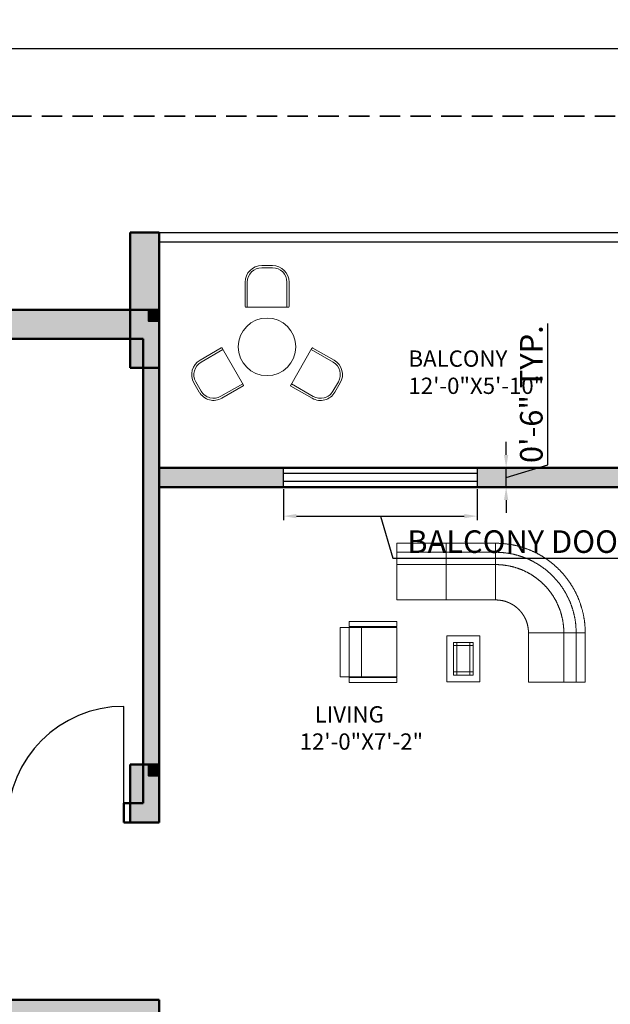
# Model space of a CAD drawing. Units: inches. Extents: x -7 to 1228, y -146 to 1091.
# Tile 57 of 88: x 193 to 376, y 786 to 1091. Entities that reach past the tile are written whole.
import ezdxf

# ---------------------------------------------------------------- set-up
doc = ezdxf.new("R2010")
doc.units = ezdxf.units.IN
doc.linetypes.add('DASHED2', pattern=[9.525, 6.35, -3.175])
for name, color, linetype, lineweight in [('A-ANNO-DIMS', 2, 'Continuous', 18), ('A-AREA-IDEN', 7, 'Continuous', 18), ('A-COLS', 6, 'Continuous', 35), ('A-DOOR', 4, 'Continuous', 25), ('A-FURN', 8, 'Continuous', 18), ('A-GLAZ', 175, 'Continuous', 25), ('A-WALL', 7, 'Continuous', 50), ('A-WALL-PATT', 251, 'Continuous', 13), ('C-PROP', 1, 'DASHED2', 35)]:
    doc.layers.add(name, color=color, linetype=linetype, lineweight=lineweight)
doc.styles.get("Standard").update_dxf_attribs({"font": 'arial.ttf'})
doc.dimstyles.new('ISO-25', dxfattribs={"dimtxt": 7, "dimasz": 4, "dimexe": 1.25, "dimexo": 0.625, "dimtad": 1, "dimdec": 1, "dimlunit": 3, "dimtxsty": 'Standard', "dimcen": 2.5, "dimadec": 0, "dimazin": 0, "dimtfac": 1, "dimtdec": 1, "dimtmove": 1, "dimatfit": 3, "dimfxl": 1, "dimarcsym": 0})

# ---------------------------------------------------------------- blocks, each defined once
blk = doc.blocks.new('A$C5EBD0AE0')
for points in [[(1613, 2118, -75), (863, 2118, -75)], [(863, 2118, -75), (863, 1980, -75)], [(1613, 1255, -75), (1613, 2118, -75)], [(2363, 2118, -75), (1613, 2118, -75)], [(1613, 2118, -75), (1613, 1980, -75)], [(2363, 2118, -75), (2371, 2118, -75), (2379, 2118, -75), (2388, 2117, -75), (2396, 2117, -75), (2404, 2117, -75), (2413, 2117, -75), (2421, 2116, -75), (2429, 2116, -75), (2438, 2116, -75), (2446, 2115, -75), (2455, 2115, -75), (2463, 2114, -75), (2471, 2113, -75), (2480, 2113, -75), (2488, 2112, -75), (2496, 2111, -75), (2504, 2110, -75), (2513, 2109, -75), (2521, 2108, -75), (2529, 2107, -75), (2538, 2106, -75), (2546, 2105, -75), (2554, 2104, -75), (2563, 2103, -75), (2571, 2102, -75), (2579, 2100, -75), (2587, 2099, -75), (2596, 2098, -75), (2604, 2096, -75), (2612, 2095, -75), (2620, 2093, -75), (2628, 2092, -75), (2637, 2090, -75), (2645, 2088, -75), (2653, 2086, -75), (2661, 2085, -75), (2669, 2083, -75), (2677, 2081, -75), (2686, 2079, -75), (2694, 2077, -75), (2702, 2075, -75), (2710, 2073, -75), (2718, 2071, -75), (2726, 2068, -75), (2734, 2066, -75), (2742, 2064, -75), (2750, 2061, -75), (2758, 2059, -75), (2766, 2057, -75), (2774, 2054, -75), (2782, 2052, -75), (2790, 2049, -75), (2798, 2046, -75), (2806, 2044, -75), (2814, 2041, -75), (2822, 2038, -75), (2829, 2035, -75), (2837, 2032, -75), (2845, 2029, -75), (2853, 2026, -75), (2861, 2023, -75), (2869, 2020, -75), (2876, 2017, -75), (2884, 2014, -75), (2892, 2011, -75), (2899, 2008, -75), (2907, 2004, -75), (2915, 2001, -75), (2922, 1997, -75), (2930, 1994, -75), (2938, 1990, -75), (2945, 1987, -75), (2953, 1983, -75), (2960, 1980, -75), (2968, 1976, -75), (2975, 1972, -75), (2983, 1968, -75), (2990, 1965, -75), (2998, 1961, -75), (3005, 1957, -75), (3012, 1953, -75), (3020, 1949, -75), (3027, 1945, -75), (3034, 1941, -75), (3041, 1937, -75), (3049, 1932, -75), (3056, 1928, -75), (3063, 1924, -75), (3070, 1920, -75), (3077, 1915, -75), (3084, 1911, -75), (3092, 1906, -75), (3099, 1902, -75), (3106, 1897, -75), (3113, 1893, -75), (3120, 1888, -75), (3127, 1883, -75), (3133, 1879, -75), (3140, 1874, -75), (3147, 1869, -75), (3154, 1864, -75), (3161, 1859, -75), (3168, 1855, -75), (3174, 1850, -75), (3181, 1845, -75), (3188, 1840, -75), (3194, 1834, -75), (3201, 1829, -75), (3207, 1824, -75), (3214, 1819, -75), (3220, 1814, -75), (3227, 1808, -75), (3233, 1803, -75), (3240, 1798, -75), (3246, 1792, -75), (3253, 1787, -75), (3259, 1781, -75), (3265, 1776, -75), (3271, 1770, -75), (3278, 1765, -75), (3284, 1759, -75), (3290, 1753, -75), (3296, 1748, -75), (3302, 1742, -75), (3308, 1736, -75), (3314, 1730, -75), (3320, 1725, -75), (3326, 1719, -75), (3332, 1713, -75), (3338, 1707, -75), (3344, 1701, -75), (3349, 1695, -75), (3355, 1689, -75), (3361, 1683, -75), (3367, 1676, -75), (3372, 1670, -75), (3378, 1664, -75), (3383, 1658, -75), (3389, 1651, -75), (3394, 1645, -75), (3400, 1639, -75), (3405, 1632, -75), (3411, 1626, -75), (3416, 1620, -75), (3421, 1613, -75), (3426, 1607, -75), (3432, 1600, -75), (3437, 1593, -75), (3442, 1587, -75), (3447, 1580, -75), (3452, 1574, -75), (3457, 1567, -75), (3462, 1560, -75), (3467, 1553, -75), (3472, 1547, -75), (3477, 1540, -75), (3481, 1533, -75), (3486, 1526, -75), (3491, 1519, -75), (3495, 1512, -75), (3500, 1505, -75), (3505, 1498, -75), (3509, 1491, -75), (3514, 1484, -75), (3518, 1477, -75), (3523, 1470, -75), (3527, 1463, -75), (3531, 1456, -75), (3536, 1448, -75), (3540, 1441, -75), (3544, 1434, -75), (3548, 1427, -75), (3552, 1419, -75), (3556, 1412, -75), (3560, 1405, -75), (3564, 1397, -75), (3568, 1390, -75), (3572, 1383, -75), (3576, 1375, -75), (3580, 1368, -75), (3583, 1360, -75), (3587, 1353, -75), (3591, 1345, -75), (3594, 1338, -75), (3598, 1330, -75), (3601, 1323, -75), (3605, 1315, -75), (3608, 1307, -75), (3612, 1300, -75), (3615, 1292, -75), (3618, 1284, -75), (3621, 1277, -75), (3625, 1269, -75), (3628, 1261, -75), (3631, 1253, -75), (3634, 1246, -75), (3637, 1238, -75), (3640, 1230, -75), (3643, 1222, -75), (3645, 1214, -75), (3648, 1206, -75), (3651, 1198, -75), (3654, 1191, -75), (3656, 1183, -75), (3659, 1175, -75), (3661, 1167, -75), (3664, 1159, -75), (3666, 1151, -75), (3669, 1143, -75), (3671, 1135, -75), (3674, 1127, -75), (3676, 1119, -75), (3678, 1111, -75), (3680, 1102, -75), (3682, 1094, -75), (3684, 1086, -75), (3686, 1078, -75), (3688, 1070, -75), (3690, 1062, -75), (3692, 1054, -75), (3694, 1046, -75), (3696, 1037, -75), (3697, 1029, -75), (3699, 1021, -75), (3701, 1013, -75), (3702, 1005, -75), (3704, 996, -75), (3705, 988, -75), (3706, 980, -75), (3708, 972, -75), (3709, 963, -75), (3710, 955, -75), (3712, 947, -75), (3713, 939, -75), (3714, 930, -75), (3715, 922, -75), (3716, 914, -75), (3717, 905, -75), (3718, 897, -75), (3719, 889, -75), (3719, 880, -75), (3720, 872, -75), (3721, 864, -75), (3721, 855, -75), (3722, 847, -75), (3723, 839, -75), (3723, 830, -75), (3723, 822, -75), (3724, 814, -75), (3724, 805, -75), (3724, 797, -75), (3725, 789, -75), (3725, 780, -75), (3725, 772, -75), (3725, 764, -75), (3725, 755, -75)], [(2363, 1255, -75), (2363, 2118, -75)], [(2363, 1255, -75), (2363, 2118, -75)], [(863, 1980, -75), (1613, 1980, -75)], [(863, 1980, -75), (863, 1793, -75)], [(1613, 1980, -75), (2363, 1980, -75)], [(1613, 1980, -75), (1613, 1793, -75)], [(2363, 1980, -75), (2370, 1980, -75), (2378, 1980, -75), (2385, 1980, -75), (2393, 1980, -75), (2400, 1980, -75), (2408, 1979, -75), (2415, 1979, -75), (2423, 1979, -75), (2430, 1978, -75), (2438, 1978, -75), (2445, 1977, -75), (2453, 1977, -75), (2460, 1976, -75), (2468, 1976, -75), (2475, 1975, -75), (2483, 1974, -75), (2490, 1974, -75), (2498, 1973, -75), (2505, 1972, -75), (2513, 1971, -75), (2520, 1970, -75), (2527, 1969, -75), (2535, 1968, -75), (2542, 1967, -75), (2550, 1966, -75), (2557, 1965, -75), (2565, 1963, -75), (2572, 1962, -75), (2579, 1961, -75), (2587, 1960, -75), (2594, 1958, -75), (2602, 1957, -75), (2609, 1955, -75), (2616, 1954, -75), (2624, 1952, -75), (2631, 1950, -75), (2638, 1949, -75), (2646, 1947, -75), (2653, 1945, -75), (2660, 1943, -75), (2668, 1942, -75), (2675, 1940, -75), (2682, 1938, -75), (2689, 1936, -75), (2697, 1934, -75), (2704, 1932, -75), (2711, 1930, -75), (2718, 1927, -75), (2725, 1925, -75), (2733, 1923, -75), (2740, 1921, -75), (2747, 1918, -75), (2754, 1916, -75), (2761, 1914, -75), (2768, 1911, -75), (2775, 1909, -75), (2782, 1906, -75), (2789, 1903, -75), (2796, 1901, -75), (2803, 1898, -75), (2810, 1895, -75), (2817, 1893, -75), (2824, 1890, -75), (2831, 1887, -75), (2838, 1884, -75), (2845, 1881, -75), (2852, 1878, -75), (2859, 1875, -75), (2866, 1872, -75), (2873, 1869, -75), (2880, 1866, -75), (2886, 1863, -75), (2893, 1859, -75), (2900, 1856, -75), (2907, 1853, -75), (2913, 1849, -75), (2920, 1846, -75), (2927, 1843, -75), (2933, 1839, -75), (2940, 1836, -75), (2947, 1832, -75), (2953, 1828, -75), (2960, 1825, -75), (2966, 1821, -75), (2973, 1817, -75), (2979, 1814, -75), (2986, 1810, -75), (2992, 1806, -75), (2999, 1802, -75), (3005, 1798, -75), (3012, 1794, -75), (3018, 1790, -75), (3024, 1786, -75), (3031, 1782, -75), (3037, 1778, -75), (3043, 1774, -75), (3049, 1770, -75), (3056, 1765, -75), (3062, 1761, -75), (3068, 1757, -75), (3074, 1752, -75), (3080, 1748, -75), (3086, 1744, -75), (3092, 1739, -75), (3098, 1735, -75), (3104, 1730, -75), (3110, 1726, -75), (3116, 1721, -75), (3122, 1716, -75), (3128, 1712, -75), (3134, 1707, -75), (3140, 1702, -75), (3146, 1697, -75), (3151, 1693, -75), (3157, 1688, -75), (3163, 1683, -75), (3168, 1678, -75), (3174, 1673, -75), (3180, 1668, -75), (3185, 1663, -75), (3191, 1658, -75), (3196, 1653, -75), (3202, 1648, -75), (3207, 1642, -75), (3213, 1637, -75), (3218, 1632, -75), (3223, 1627, -75), (3229, 1621, -75), (3234, 1616, -75), (3239, 1611, -75), (3245, 1605, -75), (3250, 1600, -75), (3255, 1594, -75), (3260, 1589, -75), (3265, 1583, -75), (3270, 1578, -75), (3275, 1572, -75), (3280, 1567, -75), (3285, 1561, -75), (3290, 1555, -75), (3295, 1550, -75), (3300, 1544, -75), (3305, 1538, -75), (3310, 1532, -75), (3314, 1527, -75), (3319, 1521, -75), (3324, 1515, -75), (3328, 1509, -75), (3333, 1503, -75), (3338, 1497, -75), (3342, 1491, -75), (3347, 1485, -75), (3351, 1479, -75), (3355, 1473, -75), (3360, 1467, -75), (3364, 1461, -75), (3368, 1454, -75), (3373, 1448, -75), (3377, 1442, -75), (3381, 1436, -75), (3385, 1430, -75), (3389, 1423, -75), (3394, 1417, -75), (3398, 1411, -75), (3402, 1404, -75), (3406, 1398, -75), (3409, 1391, -75), (3413, 1385, -75), (3417, 1379, -75), (3421, 1372, -75), (3425, 1366, -75), (3428, 1359, -75), (3432, 1352, -75), (3436, 1346, -75), (3439, 1339, -75), (3443, 1333, -75), (3446, 1326, -75), (3450, 1319, -75), (3453, 1313, -75), (3457, 1306, -75), (3460, 1299, -75), (3463, 1293, -75), (3467, 1286, -75), (3470, 1279, -75), (3473, 1272, -75), (3476, 1265, -75), (3479, 1258, -75), (3483, 1252, -75), (3486, 1245, -75), (3489, 1238, -75), (3491, 1231, -75), (3494, 1224, -75), (3497, 1217, -75), (3500, 1210, -75), (3503, 1203, -75), (3506, 1196, -75), (3508, 1189, -75), (3511, 1182, -75), (3513, 1175, -75), (3516, 1168, -75), (3519, 1161, -75), (3521, 1154, -75), (3523, 1147, -75), (3526, 1139, -75), (3528, 1132, -75), (3530, 1125, -75), (3533, 1118, -75), (3535, 1111, -75), (3537, 1104, -75), (3539, 1096, -75), (3541, 1089, -75), (3543, 1082, -75), (3545, 1075, -75), (3547, 1067, -75), (3549, 1060, -75), (3551, 1053, -75), (3553, 1046, -75), (3554, 1038, -75), (3556, 1031, -75), (3558, 1024, -75), (3559, 1016, -75), (3561, 1009, -75), (3563, 1002, -75), (3564, 994, -75), (3566, 987, -75), (3567, 979, -75), (3568, 972, -75), (3570, 965, -75), (3571, 957, -75), (3572, 950, -75), (3573, 942, -75), (3574, 935, -75), (3575, 928, -75), (3576, 920, -75), (3577, 913, -75), (3578, 905, -75), (3579, 898, -75), (3580, 890, -75), (3581, 883, -75), (3582, 875, -75), (3582, 868, -75), (3583, 860, -75), (3584, 853, -75), (3584, 845, -75), (3585, 838, -75), (3585, 830, -75), (3586, 823, -75), (3586, 815, -75), (3586, 808, -75), (3587, 800, -75), (3587, 793, -75), (3587, 785, -75), (3587, 778, -75), (3588, 770, -75), (3588, 763, -75), (3588, 755, -75)], [(863, 1793, -75), (1613, 1793, -75)], [(863, 1793, -75), (863, 1255, -75)], [(1613, 1793, -75), (1613, 1255, -75)], [(1613, 1793, -75), (2363, 1793, -75)], [(2363, 1793, -75), (2369, 1793, -75), (2375, 1793, -75), (2382, 1793, -75), (2388, 1792, -75), (2394, 1792, -75), (2401, 1792, -75), (2407, 1792, -75), (2414, 1791, -75), (2420, 1791, -75), (2426, 1791, -75), (2433, 1790, -75), (2439, 1790, -75), (2445, 1789, -75), (2452, 1789, -75), (2458, 1788, -75), (2464, 1788, -75), (2471, 1787, -75), (2477, 1786, -75), (2483, 1786, -75), (2490, 1785, -75), (2496, 1784, -75), (2502, 1783, -75), (2509, 1782, -75), (2515, 1781, -75), (2521, 1781, -75), (2527, 1780, -75), (2534, 1779, -75), (2540, 1777, -75), (2546, 1776, -75), (2553, 1775, -75), (2559, 1774, -75), (2565, 1773, -75), (2571, 1772, -75), (2577, 1770, -75), (2584, 1769, -75), (2590, 1768, -75), (2596, 1766, -75), (2602, 1765, -75), (2609, 1763, -75), (2615, 1762, -75), (2621, 1760, -75), (2627, 1758, -75), (2633, 1757, -75), (2639, 1755, -75), (2645, 1753, -75), (2652, 1752, -75), (2658, 1750, -75), (2664, 1748, -75), (2670, 1746, -75), (2676, 1744, -75), (2682, 1742, -75), (2688, 1740, -75), (2694, 1738, -75), (2700, 1736, -75), (2706, 1734, -75), (2712, 1732, -75), (2718, 1730, -75), (2724, 1728, -75), (2730, 1725, -75), (2736, 1723, -75), (2742, 1721, -75), (2748, 1719, -75), (2754, 1716, -75), (2760, 1714, -75), (2766, 1711, -75), (2771, 1709, -75), (2777, 1706, -75), (2783, 1704, -75), (2789, 1701, -75), (2795, 1698, -75), (2800, 1696, -75), (2806, 1693, -75), (2812, 1690, -75), (2818, 1688, -75), (2823, 1685, -75), (2829, 1682, -75), (2835, 1679, -75), (2840, 1676, -75), (2846, 1673, -75), (2852, 1670, -75), (2857, 1667, -75), (2863, 1664, -75), (2868, 1661, -75), (2874, 1658, -75), (2880, 1655, -75), (2885, 1652, -75), (2891, 1648, -75), (2896, 1645, -75), (2901, 1642, -75), (2907, 1638, -75), (2912, 1635, -75), (2918, 1632, -75), (2923, 1628, -75), (2928, 1625, -75), (2934, 1621, -75), (2939, 1618, -75), (2944, 1614, -75), (2950, 1611, -75), (2955, 1607, -75), (2960, 1603, -75), (2965, 1600, -75), (2970, 1596, -75), (2976, 1592, -75), (2981, 1589, -75), (2986, 1585, -75), (2991, 1581, -75), (2996, 1577, -75), (3001, 1573, -75), (3006, 1569, -75), (3011, 1565, -75), (3016, 1561, -75), (3021, 1557, -75), (3026, 1553, -75), (3031, 1549, -75), (3035, 1545, -75), (3040, 1541, -75), (3045, 1537, -75), (3050, 1532, -75), (3055, 1528, -75), (3059, 1524, -75), (3064, 1520, -75), (3069, 1515, -75), (3073, 1511, -75), (3078, 1507, -75), (3083, 1502, -75), (3087, 1498, -75), (3092, 1493, -75), (3096, 1489, -75), (3101, 1484, -75), (3105, 1480, -75), (3110, 1475, -75), (3114, 1471, -75), (3118, 1466, -75), (3123, 1461, -75), (3127, 1457, -75), (3131, 1452, -75), (3136, 1447, -75), (3140, 1442, -75), (3144, 1438, -75), (3148, 1433, -75), (3152, 1428, -75), (3156, 1423, -75), (3161, 1418, -75), (3165, 1413, -75), (3169, 1408, -75), (3173, 1404, -75), (3177, 1399, -75), (3181, 1394, -75), (3184, 1388, -75), (3188, 1383, -75), (3192, 1378, -75), (3196, 1373, -75), (3200, 1368, -75), (3203, 1363, -75), (3207, 1358, -75), (3211, 1353, -75), (3215, 1347, -75), (3218, 1342, -75), (3222, 1337, -75), (3225, 1332, -75), (3229, 1326, -75), (3232, 1321, -75), (3236, 1316, -75), (3239, 1310, -75), (3243, 1305, -75), (3246, 1299, -75), (3249, 1294, -75), (3253, 1289, -75), (3256, 1283, -75), (3259, 1278, -75), (3262, 1272, -75), (3265, 1267, -75), (3268, 1261, -75), (3272, 1255, -75), (3275, 1250, -75), (3278, 1244, -75), (3281, 1239, -75), (3284, 1233, -75), (3286, 1227, -75), (3289, 1222, -75), (3292, 1216, -75), (3295, 1210, -75), (3298, 1205, -75), (3300, 1199, -75), (3303, 1193, -75), (3306, 1187, -75), (3309, 1181, -75), (3311, 1176, -75), (3314, 1170, -75), (3316, 1164, -75), (3319, 1158, -75), (3321, 1152, -75), (3324, 1146, -75), (3326, 1140, -75), (3328, 1135, -75), (3331, 1129, -75), (3333, 1123, -75), (3335, 1117, -75), (3337, 1111, -75), (3339, 1105, -75), (3342, 1099, -75), (3344, 1093, -75), (3346, 1087, -75), (3348, 1081, -75), (3350, 1075, -75), (3352, 1069, -75), (3354, 1062, -75), (3355, 1056, -75), (3357, 1050, -75), (3359, 1044, -75), (3361, 1038, -75), (3363, 1032, -75), (3364, 1026, -75), (3366, 1020, -75), (3367, 1013, -75), (3369, 1007, -75), (3371, 1001, -75), (3372, 995, -75), (3373, 989, -75), (3375, 983, -75), (3376, 976, -75), (3378, 970, -75), (3379, 964, -75), (3380, 958, -75), (3381, 951, -75), (3383, 945, -75), (3384, 939, -75), (3385, 933, -75), (3386, 926, -75), (3387, 920, -75), (3388, 914, -75), (3389, 907, -75), (3390, 901, -75), (3391, 895, -75), (3392, 889, -75), (3392, 882, -75), (3393, 876, -75), (3394, 870, -75), (3394, 863, -75), (3395, 857, -75), (3396, 851, -75), (3396, 844, -75), (3397, 838, -75), (3397, 832, -75), (3398, 825, -75), (3398, 819, -75), (3399, 812, -75), (3399, 806, -75), (3399, 800, -75), (3399, 793, -75), (3400, 787, -75), (3400, 781, -75), (3400, 774, -75), (3400, 768, -75), (3400, 762, -75), (3400, 755, -75)], [(863, 1255, -75), (1613, 1255, -75)], [(1613, 1255, -75), (2363, 1255, -75)], [(2363, 1255, -75), (2366, 1255, -75), (2369, 1255, -75), (2372, 1255, -75), (2375, 1255, -75), (2378, 1255, -75), (2381, 1255, -75), (2384, 1255, -75), (2387, 1255, -75), (2390, 1254, -75), (2393, 1254, -75), (2396, 1254, -75), (2399, 1254, -75), (2402, 1254, -75), (2406, 1253, -75), (2409, 1253, -75), (2412, 1253, -75), (2415, 1252, -75), (2418, 1252, -75), (2421, 1252, -75), (2424, 1251, -75), (2427, 1251, -75), (2430, 1251, -75), (2433, 1250, -75), (2436, 1250, -75), (2439, 1249, -75), (2442, 1249, -75), (2445, 1248, -75), (2448, 1248, -75), (2451, 1247, -75), (2454, 1247, -75), (2457, 1246, -75), (2460, 1246, -75), (2463, 1245, -75), (2466, 1244, -75), (2469, 1244, -75), (2472, 1243, -75), (2475, 1242, -75), (2478, 1242, -75), (2481, 1241, -75), (2484, 1240, -75), (2487, 1239, -75), (2490, 1239, -75), (2493, 1238, -75), (2496, 1237, -75), (2499, 1236, -75), (2502, 1235, -75), (2505, 1235, -75), (2508, 1234, -75), (2511, 1233, -75), (2514, 1232, -75), (2517, 1231, -75), (2519, 1230, -75), (2522, 1229, -75), (2525, 1228, -75), (2528, 1227, -75), (2531, 1226, -75), (2534, 1225, -75), (2537, 1224, -75), (2540, 1223, -75), (2543, 1222, -75), (2545, 1221, -75), (2548, 1219, -75), (2551, 1218, -75), (2554, 1217, -75), (2557, 1216, -75), (2560, 1215, -75), (2562, 1214, -75), (2565, 1212, -75), (2568, 1211, -75), (2571, 1210, -75), (2574, 1209, -75), (2576, 1207, -75), (2579, 1206, -75), (2582, 1205, -75), (2585, 1203, -75), (2587, 1202, -75), (2590, 1200, -75), (2593, 1199, -75), (2596, 1198, -75), (2598, 1196, -75), (2601, 1195, -75), (2604, 1193, -75), (2606, 1192, -75), (2609, 1190, -75), (2612, 1189, -75), (2614, 1187, -75), (2617, 1186, -75), (2620, 1184, -75), (2622, 1182, -75), (2625, 1181, -75), (2628, 1179, -75), (2630, 1178, -75), (2633, 1176, -75), (2635, 1174, -75), (2638, 1173, -75), (2640, 1171, -75), (2643, 1169, -75), (2645, 1168, -75), (2648, 1166, -75), (2651, 1164, -75), (2653, 1162, -75), (2656, 1160, -75), (2658, 1159, -75), (2660, 1157, -75), (2663, 1155, -75), (2665, 1153, -75), (2668, 1151, -75), (2670, 1149, -75), (2673, 1147, -75), (2675, 1146, -75), (2677, 1144, -75), (2680, 1142, -75), (2682, 1140, -75), (2685, 1138, -75), (2687, 1136, -75), (2689, 1134, -75), (2692, 1132, -75), (2694, 1130, -75), (2696, 1128, -75), (2698, 1126, -75), (2701, 1124, -75), (2703, 1122, -75), (2705, 1119, -75), (2707, 1117, -75), (2710, 1115, -75), (2712, 1113, -75), (2714, 1111, -75), (2716, 1109, -75), (2718, 1107, -75), (2720, 1104, -75), (2723, 1102, -75), (2725, 1100, -75), (2727, 1098, -75), (2729, 1096, -75), (2731, 1093, -75), (2733, 1091, -75), (2735, 1089, -75), (2737, 1086, -75), (2739, 1084, -75), (2741, 1082, -75), (2743, 1079, -75), (2745, 1077, -75), (2747, 1075, -75), (2749, 1072, -75), (2751, 1070, -75), (2753, 1068, -75), (2755, 1065, -75), (2757, 1063, -75), (2759, 1060, -75), (2761, 1058, -75), (2762, 1056, -75), (2764, 1053, -75), (2766, 1051, -75), (2768, 1048, -75), (2770, 1046, -75), (2771, 1043, -75), (2773, 1041, -75), (2775, 1038, -75), (2777, 1036, -75), (2778, 1033, -75), (2780, 1030, -75), (2782, 1028, -75), (2783, 1025, -75), (2785, 1023, -75), (2787, 1020, -75), (2788, 1018, -75), (2790, 1015, -75), (2791, 1012, -75), (2793, 1010, -75), (2795, 1007, -75), (2796, 1004, -75), (2798, 1002, -75), (2799, 999, -75), (2801, 996, -75), (2802, 994, -75), (2804, 991, -75), (2805, 988, -75), (2806, 985, -75), (2808, 983, -75), (2809, 980, -75), (2811, 977, -75), (2812, 975, -75), (2813, 972, -75), (2815, 969, -75), (2816, 966, -75), (2817, 963, -75), (2818, 961, -75), (2820, 958, -75), (2821, 955, -75), (2822, 952, -75), (2823, 949, -75), (2825, 947, -75), (2826, 944, -75), (2827, 941, -75), (2828, 938, -75), (2829, 935, -75), (2830, 932, -75), (2831, 929, -75), (2832, 927, -75), (2833, 924, -75), (2834, 921, -75), (2835, 918, -75), (2836, 915, -75), (2837, 912, -75), (2838, 909, -75), (2839, 906, -75), (2840, 903, -75), (2841, 900, -75), (2842, 897, -75), (2843, 894, -75), (2844, 892, -75), (2844, 889, -75), (2845, 886, -75), (2846, 883, -75), (2847, 880, -75), (2848, 877, -75), (2848, 874, -75), (2849, 871, -75), (2850, 868, -75), (2850, 865, -75), (2851, 862, -75), (2852, 859, -75), (2852, 856, -75), (2853, 853, -75), (2854, 850, -75), (2854, 847, -75), (2855, 844, -75), (2855, 841, -75), (2856, 838, -75), (2856, 835, -75), (2857, 832, -75), (2857, 829, -75), (2858, 826, -75), (2858, 822, -75), (2858, 819, -75), (2859, 816, -75), (2859, 813, -75), (2860, 810, -75), (2860, 807, -75), (2860, 804, -75), (2860, 801, -75), (2861, 798, -75), (2861, 795, -75), (2861, 792, -75), (2861, 789, -75), (2862, 786, -75), (2862, 783, -75), (2862, 780, -75), (2862, 777, -75), (2862, 774, -75), (2862, 771, -75), (2862, 767, -75), (2863, 764, -75), (2863, 761, -75), (2863, 758, -75), (2863, 755, -75)], [(138, 925, -75), (863, 925, -75)], [(138, 850, -75), (138, 925, -75)], [(863, 925, -75), (863, 850, -75)], [(0, 837, -75), (0, 87, -75)], [(863, 837, -75), (0, 837, -75)], [(863, 850, -75), (138, 850, -75)], [(138, 87, -75), (138, 837, -75)], [(325, 87, -75), (325, 837, -75)], [(863, 87, -75), (863, 837, -75)], [(2863, 755, -75), (2863, 5, -75)], [(3400, 755, -75), (2863, 755, -75)], [(3400, 755, -75), (3400, 5, -75)], [(3588, 755, -75), (3400, 755, -75)], [(3588, 755, -75), (3588, 5, -75)], [(3725, 755, -75), (3588, 755, -75)], [(3725, 5, -75), (3725, 755, -75)], [(0, 87, -75), (138, 87, -75)], [(138, 87, -75), (325, 87, -75)], [(863, 75, -75), (138, 75, -75)], [(138, 75, -75), (138, 0, -75)], [(325, 87, -75), (863, 87, -75)], [(863, 0, -75), (863, 75, -75)], [(3400, 5, -75), (2863, 5, -75)], [(2863, 5, -75), (3725, 5, -75)], [(3588, 5, -75), (3400, 5, -75)], [(3725, 5, -75), (3588, 5, -75)], [(138, 0, -75), (863, 0, -75)]]:
    blk.add_polyline3d(points)
for points in [[(1623, 10), (1623, 710), (1623, 710, 25), (1623, 10, 25)], [(1623, 710), (2123, 710), (2123, 710, 25), (1623, 710, 25)], [(1723, 610, -675), (1773, 610, -675), (1773, 610), (1723, 610)], [(1773, 610, -675), (1723, 610, -675), (1723, 610), (1773, 610)], [(1723, 610, -675), (1723, 560, -675), (1723, 560), (1723, 610)], [(1773, 610, -675), (1773, 560, -675), (1773, 560), (1773, 610)], [(1773, 560, -675), (1773, 610, -675), (1773, 610), (1773, 560)], [(1973, 610, -375), (1773, 610, -375), (1773, 610, -350), (1973, 610, -350)], [(2023, 610, -675), (1973, 610, -675), (1973, 610), (2023, 610)], [(1973, 610, -675), (1973, 560, -675), (1973, 560), (1973, 610)], [(1973, 110, -375), (1973, 610, -375), (1973, 610, -350), (1973, 110, -350)], [(2023, 560, -675), (2023, 610, -675), (2023, 610), (2023, 560)], [(2123, 710), (2123, 10), (2123, 10, 25), (2123, 710, 25)], [(1723, 560, -675), (1773, 560, -675), (1773, 560), (1723, 560)], [(1723, 560, -375), (1723, 160, -375), (1723, 160, -350), (1723, 560, -350)], [(2023, 560, -375), (1773, 560, -375), (1773, 560, -350), (2023, 560, -350)], [(1773, 560, -375), (1773, 110, -375), (1773, 110, -350), (1773, 560, -350)], [(1973, 560, -675), (2023, 560, -675), (2023, 560), (1973, 560)], [(2023, 160, -375), (2023, 560, -375), (2023, 560, -350), (2023, 160, -350)], [(1723, 110, -675), (1723, 160, -675), (1723, 160), (1723, 110)], [(1723, 160, -675), (1773, 160, -675), (1773, 160), (1723, 160)], [(1723, 160, -375), (2023, 160, -375), (2023, 160, -350), (1723, 160, -350)], [(1773, 160, -675), (1773, 110, -675), (1773, 110), (1773, 160)], [(1973, 110, -675), (1973, 160, -675), (1973, 160), (1973, 110)], [(1973, 160, -675), (2023, 160, -675), (2023, 160), (1973, 160)], [(2023, 110, -675), (2023, 160, -675), (2023, 160), (2023, 110)], [(2123, 10), (1623, 10), (1623, 10, 25), (2123, 10, 25)], [(1773, 110, -675), (1723, 110, -675), (1723, 110), (1773, 110)], [(1773, 110, -375), (1973, 110, -375), (1973, 110, -350), (1773, 110, -350)], [(2023, 110, -675), (1973, 110, -675), (1973, 110), (2023, 110)]]:
    blk.add_3dface(points)
blk = doc.blocks.new('*D11')
at = {"layer": 'A-ANNO-DIMS', "color": 0, "lineweight": -2, "transparency": 16777216}
for p, q in [((0, 1061.62), (0, 1083.25)), ((4, 1082), (1183, 1082)), ((1187, 1061.62), (1187, 1083.25))]:
    blk.add_line(p, q, dxfattribs=at)
at = {"layer": 'A-ANNO-DIMS', "color": 0, "transparency": 16777216}
for points in [[(4, 1082.67), (4, 1081.33), (0, 1082)], [(1183, 1082.67), (1183, 1081.33), (1187, 1082)]]:
    blk.add_solid(points, dxfattribs=at)
at = {"layer": 'Defpoints', "color": 0, "transparency": 16777216}
for p in [(1187, 1082), (0, 1061), (1187, 1061)]:
    blk.add_point(p, dxfattribs=at)
at = {"layer": 'A-ANNO-DIMS', "color": 0, "transparency": 16777216, "insert": (593.5, 1086.2), "char_height": 7, "attachment_point": 5}
blk.add_mtext('98\'-11"', dxfattribs=at)
blk = doc.blocks.new('A$C670C3AF2')
for p, q in [((1122, 1874), (972, 1874)), ((1122, 1844), (972, 1844)), ((742, 1644), (742, 1304)), ((772, 1644), (772, 1294)), ((1322, 1294), (1322, 1644)), ((1352, 1304), (1352, 1644)), ((752, 1294), (1342, 1294)), ((409, 730), (115, 560)), ((433, 709), (130, 534)), ((718, 215), (423, 726)), ((1669, 725), (1374, 214)), ((1963, 533), (1659, 708)), ((1978, 559), (1683, 729)), ((30, 246), (105, 116)), ((56, 261), (131, 131)), ((405, 58), (708, 233)), ((420, 32), (714, 202)), ((1378, 200), (1673, 30)), ((1384, 231), (1688, 56)), ((1961, 130), (2036, 259)), ((1987, 115), (2062, 244))]:
    blk.add_line(p, q)
blk.add_circle((1046, 745), 400)
for centre, radius, start, end in [((972, 1644), 230, 90, 180), ((972, 1644), 200, 90, 180), ((1122, 1644), 230, 0, 90), ((1122, 1644), 200, 0, 90), ((752, 1304), 10, 180, 270), ((1342, 1304), 10, 270, 0), ((414, 721), 10, 30, 120), ((1678, 720), 10, 60, 150), ((230, 361), 230, 120, 210), ((1863, 359), 230, 330, 60), ((230, 361), 200, 120, 210), ((1863, 359), 200, 330, 60), ((709, 210), 10, 300, 30), ((1383, 209), 10, 150, 240), ((305, 231), 230, 210, 300), ((305, 231), 200, 210, 300), ((1788, 230), 230, 240, 330), ((1788, 230), 200, 240, 330)]:
    blk.add_arc(centre, radius, start, end)
blk = doc.blocks.new('WIN-BALCONY-60')
for p, q in [((0, 0), (0, 6)), ((0, 6), (60, 6)), ((0, 4.29), (60, 4.29)), ((60, 6), (60, 0)), ((60, 4.29), (60, 1.76)), ((60, 1.76), (0, 1.76)), ((60, 0), (0, 0))]:
    blk.add_line(p, q)
blk = doc.blocks.new('DOOR-900')
blk.add_line((36, 0), (36, 36))
blk.add_arc((36, 0), 36, 90, 180)
blk = doc.blocks.new('*D52')
at = {"layer": 'A-ANNO-DIMS', "color": 0, "lineweight": -2, "transparency": 16777216}
for p, q in [((274.55, 945.37), (274.55, 935.75)), ((334.55, 945.37), (334.55, 935.75)), ((278.55, 937), (330.55, 937)), ((304.55, 937), (308.46, 923.95)), ((308.46, 923.95), (433.58, 923.95))]:
    blk.add_line(p, q, dxfattribs=at)
at = {"layer": 'A-ANNO-DIMS', "color": 0, "transparency": 16777216}
for points in [[(278.55, 937.67), (278.55, 936.33), (274.55, 937)], [(330.55, 937.67), (330.55, 936.33), (334.55, 937)]]:
    blk.add_solid(points, dxfattribs=at)
at = {"layer": 'Defpoints', "color": 0, "transparency": 16777216}
for p in [(274.55, 946), (334.55, 946), (334.55, 937)]:
    blk.add_point(p, dxfattribs=at)
at = {"layer": 'A-ANNO-DIMS', "color": 0, "transparency": 16777216, "insert": (371.02, 928.19), "char_height": 7, "attachment_point": 5}
blk.add_mtext('BALCONY DOOR 5\'-0" TYP.', dxfattribs=at)
blk = doc.blocks.new('*D53')
at = {"layer": 'A-ANNO-DIMS', "color": 0, "lineweight": -2, "transparency": 16777216}
for p, q in [((356.46, 952.87), (356.46, 996.79)), ((343.55, 956), (343.55, 960)), ((343.55, 949), (356.46, 952.87)), ((335.17, 952), (344.8, 952)), ((343.55, 946), (343.55, 952)), ((343.55, 946), (343.55, 952)), ((335.17, 946), (344.8, 946)), ((343.55, 942), (343.55, 938))]:
    blk.add_line(p, q, dxfattribs=at)
at = {"layer": 'A-ANNO-DIMS', "color": 0, "transparency": 16777216}
for points in [[(342.88, 956), (344.21, 956), (343.55, 952)], [(342.88, 942), (344.21, 942), (343.55, 946)]]:
    blk.add_solid(points, dxfattribs=at)
at = {"layer": 'Defpoints', "color": 0, "transparency": 16777216}
for p in [(334.55, 952), (343.55, 952), (334.55, 946)]:
    blk.add_point(p, dxfattribs=at)
at = {"layer": 'A-ANNO-DIMS', "color": 0, "transparency": 16777216, "insert": (352.26, 974.83), "char_height": 7, "attachment_point": 5, "rotation": 90}
blk.add_mtext('0\'-6" TYP.', dxfattribs=at)

msp = doc.modelspace()

# ---------------------------------------------------------------- hatches: boundary and pattern name
at = {"layer": 'A-COLS'}
h = msp.add_hatch(color=256, dxfattribs=at)
h.dxf.hatch_style = 1
h.paths.add_polyline_path([(236, 997.45), (232.71, 997.45), (232.71, 1001), (227, 1001), (227, 983), (236, 983)])
h = msp.add_hatch(color=256, dxfattribs=at)
h.dxf.hatch_style = 1
h.paths.add_polyline_path([(236, 997.45), (236, 1001), (232.71, 1001), (232.71, 997.45)])
h = msp.add_hatch(color=256, dxfattribs=at)
h.dxf.hatch_style = 1
h.paths.add_polyline_path([(236, 856.45), (232.71, 856.45), (232.71, 860), (227, 860), (227, 842), (236, 842)])
h = msp.add_hatch(color=256, dxfattribs=at)
h.dxf.hatch_style = 1
h.paths.add_polyline_path([(236, 856.45), (236, 860), (232.71, 860), (232.71, 856.45)])
at = {"layer": 'A-WALL-PATT'}
h = msp.add_hatch(color=256, dxfattribs=at)
h.dxf.hatch_style = 1
h.paths.add_polyline_path([(69, 568), (60, 568), (60, 493), (63.29, 493), (69, 493)])
h.paths.add_polyline_path([(69, 662.41), (60, 662.41), (60, 586), (69, 586)], flags=17)
h.paths.add_polyline_path([(69, 723), (184, 723), (184, 734), (179, 734), (179, 728), (69, 728), (69, 741.62), (60, 741.62), (60, 698.41), (69, 698.41)], flags=17)
h.paths.add_polyline_path([(69, 782), (231, 782), (231, 728), (231, 723), (231, 586), (236, 586), (236, 787), (69, 787), (69, 800.13), (60, 800.13), (60, 765.62), (69, 765.62)])
h.paths.add_polyline_path([(184, 842), (189, 842), (189, 848), (173, 848), (173, 842), (179, 842), (179, 787), (184, 787)])
h.paths.add_polyline_path([(118.22, 69), (69, 69), (69, 60), (118.22, 60)])
h.paths.add_polyline_path([(227, 69), (154.22, 69), (154.22, 60), (227, 60)])
h.paths.add_polyline_path([(236, 60), (232.71, 60), (227, 60), (227, 36), (236, 36)])
h.paths.add_polyline_path([(389, 60), (380, 60), (380, 36), (389, 36)])
h.paths.add_polyline_path([(384, 181), (380, 181), (380, 115), (380, 78), (384, 78)])
h.paths.add_polyline_path([(380, 115), (334.55, 115), (334.55, 109), (380, 109)])
h.paths.add_polyline_path([(274.55, 115), (236, 115), (236, 201), (232.71, 201), (231, 201), (231, 78), (236, 78), (236, 109), (274.55, 109)])
h.paths.add_polyline_path([(69, 123), (60, 123), (60, 78), (69, 78)])
h.paths.add_polyline_path([(69, 201), (60, 201), (60, 159), (69, 159)])
h.paths.add_polyline_path([(143, 219), (69, 219), (69, 213), (143, 213)], flags=17)
h.paths.add_polyline_path([(189, 219), (184, 219), (184, 274), (231, 274), (231, 219), (236, 219), (236, 279), (184, 279), (184, 297), (179, 297), (179, 279), (69, 279), (69, 290.91), (60, 290.91), (60, 262.18), (69, 262.18), (69, 274), (179, 274), (179, 219), (173, 219), (173, 213), (189, 213)])
h.paths.add_polyline_path([(69, 238.18), (60, 238.18), (60, 219), (69, 219)], flags=17)
h.paths.add_polyline_path([(69, 333), (60, 333), (60, 314.91), (69, 314.91), (69, 316.96)])
h.paths.add_polyline_path([(190, 338), (184, 338), (69, 338), (69, 333), (179, 333), (179, 327), (184, 327), (184, 333.02), (190, 333.05)])
h.paths.add_polyline_path([(69, 386.81), (60, 386.81), (60, 351), (69, 351)])
h.paths.add_polyline_path([(69, 475), (60, 475), (60, 422.81), (69, 422.81)])
h.paths.add_polyline_path([(236, 475), (231, 475), (231, 351.24), (236, 351.24)])
h.paths.add_polyline_path([(384, 475), (380, 475), (380, 362), (384, 362)])
h.paths.add_polyline_path([(547, 307), (439, 307), (439, 356), (445, 356), (445, 362), (433, 362), (433, 307), (380, 307), (380, 244), (380, 241), (384, 241), (384, 301), (433, 301), (433, 277), (439, 277), (439, 301), (547, 301)])
h.paths.add_polyline_path([(547, 241), (439, 241), (439, 247), (433, 247), (433, 235), (547, 235)])
h.paths.add_polyline_path([(450, 69), (440.29, 69), (424.89, 69), (389, 69), (389, 60), (450, 60)])
h.paths.add_polyline_path([(547, 69), (486, 69), (486, 60), (547, 60)])
h.paths.add_polyline_path([(556, 148.27), (547, 148.27), (547, 78), (556, 78)])
h.paths.add_polyline_path([(556, 223), (547, 223), (547, 195), (547, 184.27), (556, 184.27)])
h.paths.add_polyline_path([(556, 311.19), (547, 311.19), (547, 273.08), (556, 273.08)])
h.paths.add_polyline_path([(556, 344), (552.71, 344), (547, 344), (547, 335.19), (556, 335.19)])
h.paths.add_polyline_path([(556, 249.08), (547, 249.08), (547, 241), (556, 241)])
h.paths.add_polyline_path([(547, 362), (475, 362), (475, 356), (547, 356)], flags=0)
h.paths.add_polyline_path([(556, 399.62), (547, 399.62), (547, 362), (556, 362)])
h.paths.add_polyline_path([(556, 475), (547, 475), (547, 435.62), (556, 435.62)])
h.paths.add_polyline_path([(547, 493), (389, 493), (389, 487), (547, 487)])
h.paths.add_polyline_path([(380, 493), (278, 493), (278, 487), (380, 487)])
h.paths.add_polyline_path([(227, 493), (69, 493), (69, 487), (227, 487)])
h.paths.add_polyline_path([(643, 122.44), (634, 122.44), (634, 78), (643, 78)])
h.paths.add_polyline_path([(702.5, 69), (692.79, 69), (677.39, 69), (643, 69), (643, 60), (702.5, 60)])
h.paths.add_polyline_path([(798, 69), (738.5, 69), (738.5, 60), (798, 60)])
h.paths.add_polyline_path([(807, 60), (803.71, 60), (798, 60), (798, 36), (807, 36)])
h.paths.add_polyline_path([(807, 109), (846.75, 109), (846.75, 115), (807, 115), (807, 159), (802, 159), (802, 78), (807, 78)])
h.paths.add_polyline_path([(807, 201), (802, 201), (802, 195), (807, 195)])
h.paths.add_polyline_path([(643, 201), (634, 201), (634, 158.44), (643, 158.44)])
h.paths.add_polyline_path([(756, 225), (751, 225), (751, 219), (643, 219), (643, 213), (756, 213)])
h.paths.add_polyline_path([(643, 240.85), (634, 240.85), (634, 219), (643, 219)])
h.paths.add_polyline_path([(643, 274), (643, 288.63), (634, 288.63), (634, 264.85), (643, 264.85)])
h.paths.add_polyline_path([(802, 279), (756, 279), (756, 297), (751, 297), (751, 279), (643, 279), (643, 274), (751, 274), (751, 255), (756, 255), (756, 274), (802, 274)])
h.paths.add_polyline_path([(807, 333), (803.71, 333), (802, 333), (802, 279), (802, 274), (802, 219), (807, 219)])
h.paths.add_polyline_path([(956, 182), (951, 182), (951, 115), (906.75, 115), (906.75, 109), (951, 109), (951, 78), (956, 78)])
h.paths.add_polyline_path([(960, 60), (951, 60), (951, 36), (960, 36)])
h.paths.add_polyline_path([(1021, 69), (1005.78, 69), (960, 69), (960, 60), (1021, 60)])
h.paths.add_polyline_path([(956, 224), (951, 224), (951, 218), (956, 218)])
h.paths.add_polyline_path([(956, 302), (1004, 302), (1004, 278), (1010, 278), (1010, 302), (1118, 302), (1118, 290.81), (1127, 290.81), (1127, 326.97), (1118, 326.97), (1118, 320.97), (1118, 307), (1010, 307), (1010, 356), (1016, 356), (1016, 362), (1004, 362), (1004, 307), (951, 307), (951, 244), (951, 242), (954.29, 242), (956, 242)])
h.paths.add_polyline_path([(643, 333), (634, 333), (634, 312.63), (643, 312.63), (643, 316.96)])
h.paths.add_polyline_path([(756, 338), (643, 338), (643, 333), (751, 333), (751, 327), (756, 327)])
h.paths.add_polyline_path([(643, 388), (634, 388), (634, 351), (643, 351)])
h.paths.add_polyline_path([(807, 357), (802, 357), (802, 351), (807, 351)])
h.paths.add_polyline_path([(807, 475), (802, 475), (802, 393), (807, 393)])
h.paths.add_polyline_path([(643, 475), (634, 475), (634, 424), (643, 424)])
h.paths.add_polyline_path([(798, 493), (643, 493), (643, 487), (798, 487)])
h.paths.add_polyline_path([(634, 493), (556, 493), (556, 487), (634, 487)])
h.paths.add_polyline_path([(813, 493), (807, 493), (807, 487), (813, 487)])
h.paths.add_polyline_path([(951, 493), (849, 493), (849, 487), (951, 487)])
h.paths.add_polyline_path([(956, 484), (951, 484), (951, 374), (956, 374)])
h.paths.add_polyline_path([(1109, 493), (969, 493), (969, 487), (1109, 487)])
h.paths.add_polyline_path([(1127, 484), (1118, 484), (1118, 450.64), (1127, 450.64)])
h.paths.add_polyline_path([(1127, 414.64), (1118, 414.64), (1118, 365), (1127, 365)])
h.paths.add_polyline_path([(1109, 362), (1046, 362), (1046, 356), (1109, 356)], flags=17)
h.paths.add_polyline_path([(1127, 356), (1123.45, 356), (1118, 356), (1118, 350.97), (1127, 350.97)], flags=0)
h.paths.add_polyline_path([(1127, 266.81), (1118, 266.81), (1118, 262.36), (1118, 242), (1127, 242)], flags=17)
h.paths.add_polyline_path([(1118, 242), (1010, 242), (1010, 248), (1004, 248), (1004, 237), (1118, 237)])
h.paths.add_polyline_path([(1127, 224), (1118, 224), (1118, 170), (1127, 170)])
h.paths.add_polyline_path([(1127, 134), (1118, 134), (1118, 78), (1127, 78)])
h.paths.add_polyline_path([(1118, 69), (1057, 69), (1057, 60), (1118, 60)])
h.paths.add_polyline_path([(227, 571.55), (227, 574), (69, 574), (69, 568), (227, 568)])
h.paths.add_polyline_path([(380, 571.55), (380, 574), (278, 574), (278, 568), (380, 568)])
h.paths.add_polyline_path([(242, 574), (236, 574), (236, 568), (242, 568)])
h.paths.add_polyline_path([(547, 571.55), (547, 574), (389, 574), (389, 568), (547, 568)])
h.paths.add_polyline_path([(384, 733), (380, 733), (380, 586), (384, 586)])
h.paths.add_polyline_path([(556, 646), (634, 646), (634, 655), (547, 655), (547, 586), (556, 586)])
h.paths.add_polyline_path([(634, 574), (556, 574), (556, 568), (634, 568)])
h.paths.add_polyline_path([(643, 655), (634, 655), (634, 586), (643, 586)])
h.paths.add_polyline_path([(798, 574), (643, 574), (643, 568), (798, 568)])
h.paths.add_polyline_path([(643, 663.85), (634, 663.85), (634, 655), (643, 655)])
h.paths.add_polyline_path([(556, 676.97), (547, 676.97), (547, 655), (556, 655)])
h.paths.add_polyline_path([(556, 733), (547, 733), (547, 712.97), (556, 712.97)])
h.paths.add_polyline_path([(643, 710), (634, 710), (634, 699.85), (643, 699.85)])
h.paths.add_polyline_path([(807, 668), (802, 668), (802, 586), (807, 586)])
h.paths.add_polyline_path([(951, 574), (849, 574), (849, 568), (951, 568)])
h.paths.add_polyline_path([(956, 691), (951, 691), (951, 577), (956, 577)])
h.paths.add_polyline_path([(1109, 574), (969, 574), (969, 568), (1109, 568)])
h.paths.add_polyline_path([(1127, 643.4), (1118, 643.4), (1118, 577), (1127, 577)])
h.paths.add_polyline_path([(1127, 568), (1123.45, 568), (1118, 568), (1118, 493), (1127, 493)])
h.paths.add_polyline_path([(1127, 733), (1118, 733), (1118, 679.4), (1127, 679.4)])
h.paths.add_polyline_path([(1127, 777.35), (1118, 777.35), (1118, 770.04), (1118, 751), (1127, 751)], flags=17)
h.paths.add_polyline_path([(1118, 751), (1010, 751), (1010, 757), (1004, 757), (1004, 745), (1118, 745)])
h.paths.add_polyline_path([(956, 811), (1004, 811), (1004, 787), (1010, 787), (1010, 811), (1017.87, 811), (1017.87, 811.63, -0.414214), (1018.25, 812), (1031.98, 812, -0.414214), (1032.35, 811.63), (1032.35, 811), (1118, 811), (1118, 801.35), (1127, 801.35), (1127, 834.69), (1118, 834.69), (1118, 830.24), (1118, 817), (1010, 817), (1010, 866), (1016, 866), (1016, 872), (1004, 872), (1004, 817), (956, 817), (956, 866), (951, 866), (951, 751), (954.29, 751), (956, 751)])
h.paths.add_polyline_path([(1118, 872), (1046, 872), (1046, 866), (1118, 866)], flags=17)
h.paths.add_polyline_path([(1127, 924.71), (1118, 924.71), (1118, 884), (1127, 884)])
h.paths.add_polyline_path([(1127, 866), (1123.71, 866), (1118, 866), (1118, 858.69), (1127, 858.69)], flags=17)
h.paths.add_polyline_path([(956, 983), (951, 983), (951, 952), (807, 952), (807, 983), (802, 983), (802, 902), (807, 902), (807, 946), (951, 946), (951, 884), (956, 884)])
h.paths.add_polyline_path([(807, 842), (802, 842), (802, 787), (756, 787), (756, 806), (751, 806), (751, 787), (643, 787), (643, 782), (751, 782), (751, 764), (756, 764), (756, 782), (802, 782), (802, 728), (807, 728)])
h.paths.add_polyline_path([(756, 848), (643, 848), (643, 842), (751, 842), (751, 836), (756, 836)])
h.paths.add_polyline_path([(756, 734), (751, 734), (751, 728), (643, 728), (643, 723), (756, 723)])
h.paths.add_polyline_path([(643, 749.79), (634, 749.79), (634, 728), (637.29, 728), (643, 728)])
h.paths.add_polyline_path([(643, 805.41), (634, 805.41), (634, 773.79), (643, 773.79)])
h.paths.add_polyline_path([(643, 896.66), (634, 896.66), (634, 860), (637.29, 860), (643, 860)])
h.paths.add_polyline_path([(643, 842), (634, 842), (634, 829.41), (643, 829.41)])
h.paths.add_polyline_path([(643, 983), (634, 983), (634, 932.66), (643, 932.66)])
h.paths.add_polyline_path([(1127, 983), (1118, 983), (1118, 960.71), (1127, 960.71)])
h.paths.add_polyline_path([(1118, 1001), (1077.53, 1001), (1077.53, 992), (1118, 992)])
h.paths.add_polyline_path([(1041.53, 1001), (960, 1001), (960, 992), (1041.53, 992)])
h.paths.add_polyline_path([(960, 1025), (951, 1025), (951, 1001), (954.29, 1001), (960, 1001)])
h.paths.add_polyline_path([(807, 1025), (798, 1025), (798, 1001), (807, 1001)])
h.paths.add_polyline_path([(798, 1001), (738.5, 1001), (738.5, 992), (798, 992)])
h.paths.add_polyline_path([(702.5, 1001), (643, 1001), (643, 992), (702.5, 992)])
h.paths.add_polyline_path([(547, 1001), (499.11, 1001), (499.11, 992), (547, 992)])
h.paths.add_polyline_path([(463.11, 1001), (389, 1001), (389, 992), (463.11, 992)])
h.paths.add_polyline_path([(389, 1025), (380, 1025), (380, 1022), (380, 1001), (383.29, 1001), (389, 1001)])
h.paths.add_polyline_path([(236, 1025), (227, 1025), (227, 1001), (236, 1001)])
h.paths.add_polyline_path([(236, 983), (231, 983), (231, 860), (236, 860)])
h.paths.add_polyline_path([(274.55, 952), (236, 952), (236, 946), (274.55, 946)])
h.paths.add_polyline_path([(380, 952), (334.55, 952), (334.55, 946), (380, 946)])
h.paths.add_polyline_path([(384, 983), (380, 983), (380, 884), (383.29, 884), (384, 884)])
h.paths.add_polyline_path([(227, 1001), (155.01, 1001), (155.01, 992), (162.87, 992), (227, 992)])
h.paths.add_polyline_path([(119.01, 1001), (69, 1001), (69, 992), (119.01, 992)])
h.paths.add_polyline_path([(69, 983), (60, 983), (60, 922.99), (69, 922.99)])
h.paths.add_polyline_path([(69, 886.99), (60, 886.99), (60, 860), (63.29, 860), (69, 860)])
h.paths.add_polyline_path([(143, 848), (69, 848), (69, 842), (143, 842)])

# ---------------------------------------------------------------- linework, layer by layer
at = {"layer": 'A-COLS'}
for points in [[(236, 1001), (232.71, 1001), (232.71, 997.45), (236, 997.45)], [(236, 860), (232.71, 860), (232.71, 856.45), (236, 856.45)]]:
    msp.add_lwpolyline(points, close=True, dxfattribs=at)
at = {"layer": 'A-GLAZ'}
for p, q in [((236, 1025), (380, 1025)), ((380, 1022), (236, 1022))]:
    msp.add_line(p, q, dxfattribs=at)
at = {"layer": 'A-WALL'}
for p, q in [((236, 1025), (227, 1025)), ((227, 1025), (227, 992)), ((236, 1001), (236, 1025)), ((236, 1001), (60, 1001)), ((236, 1001), (227, 1001)), ((227, 1001), (227, 983)), ((236, 992), (236, 1001)), ((236, 1001), (236, 1001)), ((236, 983), (236, 1001)), ((231, 992), (69, 992)), ((231, 992), (231, 848)), ((236, 992), (236, 842)), ((227, 983), (236, 983)), ((380, 952), (236, 952)), ((380, 946), (236, 946)), ((236, 860), (227, 860)), ((227, 860), (227, 842)), ((236, 842), (236, 860)), ((231, 848), (225, 848)), ((225, 848), (225, 842)), ((236, 842), (225, 842)), ((227, 842), (236, 842)), ((236, 787), (69, 787)), ((236, 787), (236, 574))]:
    msp.add_line(p, q, dxfattribs=at)
at = {"layer": 'C-PROP'}
msp.add_line((1187, 1061), (0, 1061), dxfattribs=at)

# ---------------------------------------------------------------- block references
at = {"layer": 'A-DOOR'}
msp.add_blockref('DOOR-900', (189, 842), dxfattribs=at)
at = {"layer": 'A-FURN'}
for name, p, xscale, yscale, zscale in [('A$C670C3AF2', (246.08, 972.87), 0.022327308386288, 0.022327308386288, 0.022327308386288), ('A$C5EBD0AE0', (292.12, 885.43, 1.53), 0.0203846211271561, 0.0203846211271561, 0.0203846211271561)]:
    msp.add_blockref(name, p, dxfattribs=dict(at, xscale=xscale, yscale=yscale, zscale=zscale))
at = {"layer": 'A-GLAZ'}
msp.add_blockref('WIN-BALCONY-60', (274.55, 946), dxfattribs=at)

# ---------------------------------------------------------------- texts
at = {"layer": 'A-AREA-IDEN', "char_height": 5.0568, "attachment_point": 1}
for s, insert in [('BALCONY\\P12\'-0"X5\'-10"', (313.27, 988.39)), ('   LIVING\\P12\'-0"X7\'-2"', (279.54, 878.05))]:
    msp.add_mtext_dynamic_manual_height_columns(s, width=137.2821, gutter_width=25.28, heights=[0], dxfattribs=dict(at, insert=insert))

# ---------------------------------------------------------------- dimensions: what is measured, and where the dimension line sits
at = {"layer": 'A-ANNO-DIMS'}
dim = msp.add_linear_dim(base=(1187, 1082), p1=(0, 1061), p2=(1187, 1061), dimstyle='ISO-25', override={"dimclrd": 0, "dimclre": 0, "dimclrt": 0}, dxfattribs=at)
dim.commit()
dim.dimension.update_dxf_attribs({"geometry": '*D11', "text_midpoint": (593.5, 1086.2)})
dim = msp.add_linear_dim(base=(343.55, 952), p1=(334.55, 946), p2=(334.55, 952), angle=90, text='<> TYP.', dimstyle='ISO-25', override={"dimdec": 1, "dimlfac": 1, "dimrnd": 0, "dimzin": 1, "dimdsep": 46, "dimlunit": 4, "dimfrac": 2}, dxfattribs=at)
dim.commit()
dim.dimension.update_dxf_attribs({"geometry": '*D53', "text_midpoint": (352.26, 953.5)})
dim = msp.add_linear_dim(base=(334.55, 937), p1=(274.55, 946), p2=(334.55, 946), text='BALCONY DOOR <> TYP.', dimstyle='ISO-25', override={"dimdec": 1, "dimlfac": 1, "dimrnd": 0, "dimzin": 1, "dimdsep": 46, "dimlunit": 4, "dimfrac": 2}, dxfattribs=at)
dim.commit()
dim.dimension.update_dxf_attribs({"geometry": '*D52', "text_midpoint": (309.09, 928.19)})

doc.saveas('drawing.dxf')
